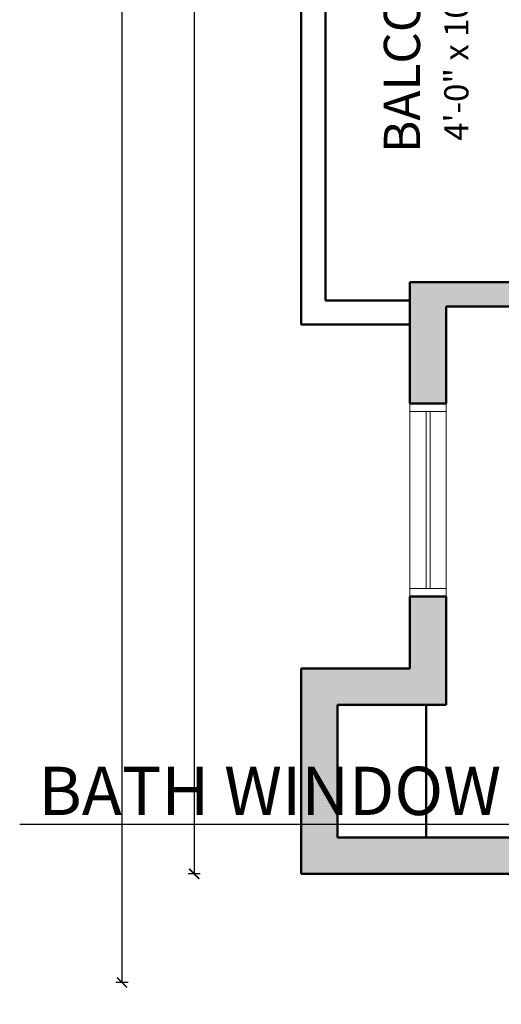
# Model space of a CAD drawing. Units: inches. Extents: x 375 to 1122, y 27 to 1069.
# Tile 2 of 155: x 375 to 494, y 155 to 400. Entities that reach past the tile are written whole.
import ezdxf

# ---------------------------------------------------------------- set-up
doc = ezdxf.new("R2010")
doc.units = ezdxf.units.IN
for name, color, linetype, lineweight in [('A-ANNO-DIMS', 2, 'Continuous', 18), ('A-AREA-IDEN', 7, 'Continuous', 18), ('A-WALL-PATT', 252, 'Continuous', 13), ('Walls', 250, 'Continuous', 50), ('Windows', 122, 'Continuous', 18)]:
    doc.layers.add(name, color=color, linetype=linetype, lineweight=lineweight)
doc.styles.get("Standard").update_dxf_attribs({"font": 'arial.ttf'})
doc.dimstyles.new('ISO-25', dxfattribs={"dimtxt": 12, "dimasz": 2.5, "dimexe": 1.5, "dimexo": 1.5, "dimtad": 1, "dimdec": 1, "dimlunit": 3, "dimtxsty": 'Standard', "dimblk": 'ARCHTICK', "dimcen": 2.5, "dimadec": 0, "dimazin": 0, "dimtfac": 1, "dimtdec": 1, "dimtmove": 0, "dimatfit": 3, "dimfxl": 1.5, "dimfxlon": 1, "dimarcsym": 0})

# ---------------------------------------------------------------- blocks, each defined once
blk = doc.blocks.new('_ArchTick')
at = {"color": 0, "linetype": 'ByBlock', "const_width": 0.15}
blk.add_lwpolyline([(-0.5, -0.5), (0.5, 0.5)], dxfattribs=at)
blk = doc.blocks.new('*D28')
at = {"layer": 'A-ANNO-DIMS', "color": 0, "lineweight": -2, "transparency": 16777216}
for p, q in [((419.42, 982.53), (416.42, 982.53)), ((417.92, 982.53), (417.92, 187.53)), ((419.42, 187.53), (416.42, 187.53))]:
    blk.add_line(p, q, dxfattribs=at)
at = {"layer": 'Defpoints', "color": 0, "transparency": 16777216}
for p in [(444.51, 982.53), (417.92, 187.53), (444.51, 187.53)]:
    blk.add_point(p, dxfattribs=at)
at = {"layer": 'A-ANNO-DIMS', "color": 0, "lineweight": -2, "transparency": 16777216, "xscale": 2.5, "yscale": 2.5, "zscale": 2.5}
for p, rotation in [((417.92, 982.53), 90), ((417.92, 187.53), 270)]:
    blk.add_blockref('_ArchTick', p, dxfattribs=dict(at, rotation=rotation))
at = {"layer": 'A-ANNO-DIMS', "color": 0, "transparency": 16777216, "insert": (411.17, 585.03), "char_height": 12, "attachment_point": 5, "rotation": 90}
blk.add_mtext('66\'-3"', dxfattribs=at)
blk = doc.blocks.new('WINDOW-48IN')
for p, q in [((2, 5), (46, 5)), ((2, 4), (46, 4))]:
    blk.add_line(p, q)
blk.add_lwpolyline([(48, 0), (0, 0), (0, 9), (48, 9)], close=True)
for points in [[(2, 0), (2, 9)], [(46, 9), (46, 0)]]:
    blk.add_lwpolyline(points)
blk = doc.blocks.new('*D49')
at = {"layer": 'A-ANNO-DIMS', "color": 0, "lineweight": -2, "transparency": 16777216}
for p, q in [((606.51, 198.25), (606.51, 201.25)), ((628.01, 198.25), (628.01, 201.25)), ((606.51, 199.75), (374.6, 199.75)), ((628.01, 199.75), (606.51, 199.75))]:
    blk.add_line(p, q, dxfattribs=at)
at = {"layer": 'Defpoints', "color": 0, "transparency": 16777216}
for p in [(606.51, 199.75), (606.51, 196.53), (628.01, 196.53)]:
    blk.add_point(p, dxfattribs=at)
at = {"layer": 'A-ANNO-DIMS', "color": 0, "lineweight": -2, "transparency": 16777216, "xscale": 2.5, "yscale": 2.5, "zscale": 2.5, "rotation": 180}
blk.add_blockref('_ArchTick', (606.51, 199.75), dxfattribs=at)
at = {"layer": 'A-ANNO-DIMS', "color": 0, "lineweight": -2, "transparency": 16777216, "xscale": 2.5, "yscale": 2.5, "zscale": 2.5}
blk.add_blockref('_ArchTick', (628.01, 199.75), dxfattribs=at)
at = {"layer": 'A-ANNO-DIMS', "color": 0, "transparency": 16777216, "insert": (489.3, 206.59), "char_height": 12, "attachment_point": 5}
blk.add_mtext('BATH WINDOW 1\'-9 1/2" TYP.', dxfattribs=at)
blk = doc.blocks.new('*D71')
at = {"layer": 'A-ANNO-DIMS', "color": 0, "lineweight": -2, "transparency": 16777216}
for p, q in [((520.11, 444.53), (520.11, 661.17)), ((518.61, 444.53), (521.61, 444.53)), ((520.11, 360.53), (520.11, 444.53)), ((518.61, 360.53), (521.61, 360.53))]:
    blk.add_line(p, q, dxfattribs=at)
at = {"layer": 'Defpoints', "color": 0, "transparency": 16777216}
for p in [(507.51, 444.53), (520.11, 444.53), (507.51, 360.53)]:
    blk.add_point(p, dxfattribs=at)
at = {"layer": 'A-ANNO-DIMS', "color": 0, "lineweight": -2, "transparency": 16777216, "xscale": 2.5, "yscale": 2.5, "zscale": 2.5}
for p, rotation in [((520.11, 444.53), 90), ((520.11, 360.53), 270)]:
    blk.add_blockref('_ArchTick', p, dxfattribs=dict(at, rotation=rotation))
at = {"layer": 'A-ANNO-DIMS', "color": 0, "transparency": 16777216, "insert": (513.27, 554.1), "char_height": 12, "attachment_point": 5, "rotation": 90}
blk.add_mtext('3-PANEL SLIDER 7\'-0" TYP.', dxfattribs=at)
blk = doc.blocks.new('*D81')
at = {"layer": 'A-ANNO-DIMS', "color": 0, "lineweight": -2, "transparency": 16777216}
for p, q in [((444.51, 117.53), (444.51, 114.53)), ((989.01, 117.53), (989.01, 114.53)), ((444.51, 116.03), (989.01, 116.03))]:
    blk.add_line(p, q, dxfattribs=at)
at = {"layer": 'Defpoints', "color": 0, "transparency": 16777216}
for p in [(444.51, 187.53), (989.01, 187.53), (989.01, 116.03)]:
    blk.add_point(p, dxfattribs=at)
at = {"layer": 'A-ANNO-DIMS', "color": 0, "lineweight": -2, "transparency": 16777216, "xscale": 2.5, "yscale": 2.5, "zscale": 2.5, "rotation": 180}
blk.add_blockref('_ArchTick', (444.51, 116.03), dxfattribs=at)
at = {"layer": 'A-ANNO-DIMS', "color": 0, "lineweight": -2, "transparency": 16777216, "xscale": 2.5, "yscale": 2.5, "zscale": 2.5}
blk.add_blockref('_ArchTick', (989.01, 116.03), dxfattribs=at)
at = {"layer": 'A-ANNO-DIMS', "color": 0, "transparency": 16777216, "insert": (716.76, 122.86), "char_height": 12, "attachment_point": 5}
blk.add_mtext('45\'-4 1/2"', dxfattribs=at)
blk = doc.blocks.new('*D82')
at = {"layer": 'A-ANNO-DIMS', "color": 0, "lineweight": -2, "transparency": 16777216}
for p, q in [((401.51, 1009.53), (398.51, 1009.53)), ((400.01, 160.53), (400.01, 1009.53)), ((401.51, 160.53), (398.51, 160.53))]:
    blk.add_line(p, q, dxfattribs=at)
at = {"layer": 'Defpoints', "color": 0, "transparency": 16777216}
for p in [(400.01, 1009.53), (630.53, 1009.53), (630.53, 160.53)]:
    blk.add_point(p, dxfattribs=at)
at = {"layer": 'A-ANNO-DIMS', "color": 0, "lineweight": -2, "transparency": 16777216, "xscale": 2.5, "yscale": 2.5, "zscale": 2.5}
for p, rotation in [((400.01, 1009.53), 90), ((400.01, 160.53), 270)]:
    blk.add_blockref('_ArchTick', p, dxfattribs=dict(at, rotation=rotation))
at = {"layer": 'A-ANNO-DIMS', "color": 0, "transparency": 16777216, "insert": (393.26, 585.03), "char_height": 12, "attachment_point": 5, "rotation": 90}
blk.add_mtext('70\'-9"', dxfattribs=at)

msp = doc.modelspace()

# ---------------------------------------------------------------- hatches: boundary and pattern name
at = {"layer": 'A-WALL-PATT'}
h = msp.add_hatch(color=256, dxfattribs=at)
h.dxf.hatch_style = 1
h.paths.add_polyline_path([(962.01, 388.53), (989.01, 388.53), (989.01, 394.53), (962.01, 394.53), (932.01, 394.53), (932.01, 397.53), (923.01, 397.53), (923.01, 394.53), (842.01, 394.53), (842.01, 334.53), (839.51, 334.53), (839.51, 328.53), (854.01, 328.53), (854.01, 334.53), (848.01, 334.53), (848.01, 388.53), (953.01, 388.53), (953.01, 356.08), (962.01, 356.08), (962.01, 358.55), (989.01, 358.55), (989.01, 364.55), (962.01, 364.55)])
h.paths.add_polyline_path([(989.01, 502.53), (932.01, 502.53), (932.01, 583.53), (932.01, 593.53), (923.01, 593.53), (923.01, 583.53), (854.01, 583.53), (854.01, 556.53), (863.01, 556.53), (863.01, 574.53), (923.01, 574.53), (923.01, 502.53), (863.01, 502.53), (863.01, 520.53), (854.01, 520.53), (854.01, 502.53), (773.01, 502.53), (773.01, 493.53), (788.01, 493.53), (788.01, 402.03), (722.01, 402.03), (722.01, 373.53), (728.01, 373.53), (728.01, 396.03), (788.01, 396.03), (788.01, 373.53), (794.01, 373.53), (794.01, 430.53), (814.01, 430.53), (814.01, 436.53), (794.01, 436.53), (794.01, 493.53), (923.01, 493.53), (923.01, 487.53), (932.01, 487.53), (932.01, 493.53), (983.01, 493.53), (983.01, 473.53), (989.01, 473.53)])
h.paths.add_polyline_path([(797.01, 325.53), (805.01, 325.53), (805.01, 328.53), (807.51, 328.53), (807.51, 334.53), (791.01, 334.53), (791.01, 226.53), (770.76, 226.53), (770.76, 217.53), (791.01, 217.53), (791.01, 187.53), (855.01, 187.53), (855.01, 196.53), (797.01, 196.53)])
h.paths.add_polyline_path([(989.01, 238.53), (962.01, 238.53), (962.01, 256.42), (953.01, 256.42), (953.01, 229.53), (980.01, 229.53), (980.01, 196.53), (915.01, 196.53), (915.01, 187.53), (989.01, 187.53)])
h.paths.add_polyline_path([(962.01, 334.53), (884.01, 334.53), (884.01, 328.53), (918.01, 328.53), (918.01, 325.53), (932.01, 325.53), (932.01, 328.53), (953.01, 328.53), (953.01, 304.42), (962.01, 304.42)])
h.paths.add_polyline_path([(606.51, 283.53), (609.51, 283.53), (609.51, 289.53), (600.51, 289.53), (600.51, 196.53), (578.51, 196.53), (578.51, 187.53), (606.51, 187.53), (606.51, 196.53)])
h.paths.add_polyline_path([(666.51, 292.53), (660.51, 292.53), (660.51, 289.53), (633.51, 289.53), (633.51, 283.53), (660.51, 283.53), (660.51, 196.53), (628.01, 196.53), (628.01, 187.53), (630.53, 187.53), (630.53, 160.53), (636.53, 160.53), (636.53, 187.53), (660.51, 187.53), (660.51, 160.53), (666.51, 160.53), (666.51, 217.53), (686.76, 217.53), (686.76, 226.53), (666.51, 226.53)])
h.paths.add_polyline_path([(480.51, 256.42), (471.51, 256.42), (471.51, 238.53), (444.51, 238.53), (444.51, 187.53), (518.51, 187.53), (518.51, 196.53), (453.51, 196.53), (453.51, 229.53), (480.51, 229.53)])
h.paths.add_polyline_path([(480.51, 328.53), (652.51, 328.53), (652.51, 325.53), (660.51, 325.53), (660.51, 322.53), (666.51, 322.53), (666.51, 334.53), (507.51, 334.53), (507.51, 360.53), (498.51, 360.53), (498.51, 334.53), (471.51, 334.53), (471.51, 304.42), (480.51, 304.42)])
h.paths.add_polyline_path([(507.51, 484.53), (498.51, 484.53), (498.51, 444.53), (507.51, 444.53), (507.51, 454.53), (621.51, 454.53), (621.51, 460.53), (507.51, 460.53)])
h.paths.add_polyline_path([(672.51, 604.53), (683.26, 604.53), (683.26, 613.53), (669.51, 613.53), (669.51, 649.53), (663.51, 649.53), (663.51, 589.53), (507.51, 589.53), (507.51, 613.53), (498.51, 613.53), (498.51, 556.53), (507.51, 556.53), (507.51, 580.53), (663.51, 580.53), (663.51, 520.53), (669.51, 520.53), (669.51, 556.53), (683.26, 556.53), (683.26, 565.53), (672.51, 565.53)])
h.paths.add_polyline_path([(731.01, 667.53), (734.01, 667.53), (734.01, 676.53), (728.01, 676.53), (728.01, 715.53), (657.51, 715.53), (657.51, 709.53), (663.51, 709.53), (663.51, 673.53), (669.51, 673.53), (669.51, 709.53), (722.01, 709.53), (722.01, 613.53), (704.76, 613.53), (704.76, 604.53), (722.01, 604.53), (722.01, 565.53), (704.76, 565.53), (704.76, 556.53), (722.01, 556.53), (722.01, 502.53), (722.01, 460.53), (669.51, 460.53), (669.51, 496.53), (663.51, 496.53), (663.51, 460.53), (657.51, 460.53), (657.51, 454.53), (728.01, 454.53), (728.01, 493.53), (734.01, 493.53), (734.01, 502.53), (731.01, 502.53)])
h.paths.add_polyline_path([(986.01, 718.53), (959.01, 718.53), (959.01, 727.53), (950.01, 727.53), (950.01, 709.53), (977.01, 709.53), (977.01, 676.53), (794.01, 676.53), (794.01, 805.53), (802.01, 805.53), (802.01, 808.53), (804.51, 808.53), (804.51, 814.53), (788.01, 814.53), (788.01, 774.03), (728.01, 774.03), (728.01, 796.53), (722.01, 796.53), (722.01, 768.03), (788.01, 768.03), (788.01, 676.53), (773.01, 676.53), (773.01, 667.53), (923.01, 667.53), (923.01, 657.53), (932.01, 657.53), (932.01, 667.53), (986.01, 667.53)])
h.paths.add_polyline_path([(621.51, 715.53), (507.51, 715.53), (507.51, 733.53), (498.51, 733.53), (498.51, 715.53), (498.51, 685.53), (507.51, 685.53), (507.51, 709.53), (621.51, 709.53)])
h.paths.add_polyline_path([(666.51, 847.03), (660.51, 847.03), (660.51, 844.53), (652.51, 844.53), (652.51, 841.53), (480.51, 841.53), (480.51, 859.53), (471.51, 859.53), (471.51, 835.53), (498.51, 835.53), (498.51, 817.53), (507.51, 817.53), (507.51, 835.53), (666.51, 835.53)])
h.paths.add_polyline_path([(480.51, 940.53), (453.51, 940.53), (453.51, 973.53), (518.51, 973.53), (518.51, 982.53), (444.51, 982.53), (444.51, 931.53), (471.51, 931.53), (471.51, 907.53), (480.51, 907.53)])
h.paths.add_polyline_path([(606.51, 982.53), (578.51, 982.53), (578.51, 973.53), (600.51, 973.53), (600.51, 880.53), (609.51, 880.53), (609.51, 886.53), (606.51, 886.53)])
h.paths.add_polyline_path([(666.51, 943.53), (686.76, 943.53), (686.76, 952.53), (666.51, 952.53), (666.51, 1009.53), (660.51, 1009.53), (660.51, 982.53), (636.53, 982.53), (636.53, 1009.53), (630.53, 1009.53), (630.53, 982.53), (628.01, 982.53), (628.01, 973.53), (660.51, 973.53), (660.51, 886.53), (633.51, 886.53), (633.51, 880.53), (660.51, 880.53), (660.51, 877.03), (666.51, 877.03)])
h.paths.add_polyline_path([(986.01, 874.53), (932.01, 874.53), (932.01, 877.53), (923.01, 877.53), (923.01, 874.53), (788.01, 874.53), (788.01, 868.53), (788.01, 844.53), (794.01, 844.53), (794.01, 868.53), (839.01, 868.53), (839.01, 814.53), (836.51, 814.53), (836.51, 808.53), (851.01, 808.53), (851.01, 814.53), (845.01, 814.53), (845.01, 868.53), (986.01, 868.53)])
h.paths.add_polyline_path([(959.01, 838.55), (986.01, 838.55), (986.01, 844.55), (959.01, 844.55), (959.01, 847.03), (950.01, 847.03), (950.01, 814.53), (881.01, 814.53), (881.01, 808.53), (918.01, 808.53), (918.01, 805.53), (932.01, 805.53), (932.01, 808.53), (950.01, 808.53), (950.01, 793.53), (959.01, 793.53)])
h.paths.add_polyline_path([(986.01, 982.53), (899.01, 982.53), (899.01, 973.53), (923.01, 973.53), (923.01, 967.53), (932.01, 967.53), (932.01, 973.53), (980.01, 973.53), (980.01, 953.53), (986.01, 953.53)])
h.paths.add_polyline_path([(851.01, 982.53), (788.01, 982.53), (788.01, 952.53), (770.76, 952.53), (770.76, 943.53), (788.01, 943.53), (788.01, 910.53), (814.01, 910.53), (814.01, 916.53), (794.01, 916.53), (794.01, 973.53), (851.01, 973.53)])

# ---------------------------------------------------------------- linework, layer by layer
at = {"layer": 'Walls'}
for p, q in [((444.51, 324.03), (444.51, 465.03)), ((450.51, 330.03), (450.51, 459.03)), ((471.51, 334.53), (498.51, 334.53)), ((471.51, 304.42), (471.51, 334.53)), ((450.51, 330.03), (471.51, 330.03)), ((480.51, 328.53), (652.51, 328.53)), ((480.51, 304.42), (480.51, 328.53)), ((444.51, 324.03), (471.51, 324.03)), ((480.51, 304.42), (471.51, 304.42)), ((471.51, 238.53), (471.51, 256.42)), ((480.51, 256.42), (471.51, 256.42)), ((480.51, 229.53), (480.51, 256.42)), ((444.51, 187.53), (444.51, 238.53)), ((444.51, 238.53), (471.51, 238.53)), ((453.51, 229.53), (480.51, 229.53)), ((453.51, 196.53), (453.51, 229.53)), ((475.51, 196.53), (475.51, 229.53)), ((518.51, 196.53), (453.51, 196.53)), ((444.51, 187.53), (518.51, 187.53))]:
    msp.add_line(p, q, dxfattribs=at)

# ---------------------------------------------------------------- block references
at = {"layer": 'Windows', "rotation": 270}
msp.add_blockref('WINDOW-48IN', (471.51, 304.42), dxfattribs=at)

# ---------------------------------------------------------------- texts
at = {"layer": 'A-AREA-IDEN', "insert": (465.03, 360.85), "char_height": 12, "attachment_point": 1, "rotation": 90}
msp.add_mtext_dynamic_manual_height_columns('\\pxqc;{\\fArial|b1|i0|c0|p34;\\H0.75x;BALCONY\\H1.33333x;\\P\\fArial|b0|i0|c0|p34;\\H0.5x;4\'-0" x 10\'-9"}', width=66.1169, gutter_width=12.5, heights=[0], dxfattribs=at)

# ---------------------------------------------------------------- dimensions: what is measured, and where the dimension line sits
at = {"layer": 'A-ANNO-DIMS'}
for base, p1, p2, override, picture, middle in [((400.01, 1009.53), (630.53, 160.53), (630.53, 1009.53), {"dimdec": 1, "dimlfac": 1, "dimrnd": 0, "dimzin": 1, "dimdsep": 46, "dimlunit": 4, "dimfrac": 2}, '*D82', (393.26, 585.03)), ((417.92, 187.53), (444.51, 982.53), (444.51, 187.53), {"dimclrd": 0, "dimclre": 0, "dimclrt": 0}, '*D28', (411.17, 585.03))]:
    dim = msp.add_linear_dim(base=base, p1=p1, p2=p2, angle=90, dimstyle='ISO-25', override=override, dxfattribs=at)
    dim.commit()
    dim.dimension.update_dxf_attribs({"geometry": picture, "text_midpoint": middle})
for base, p1, p2, angle, text, picture, middle in [((520.11, 444.53), (507.51, 360.53), (507.51, 444.53), 90, '3-PANEL SLIDER <> TYP.', '*D71', (513.27, 554.1)), ((606.51, 199.75), (628.01, 196.53), (606.51, 196.53), 180, 'BATH WINDOW <> TYP.', '*D49', (489.3, 206.59))]:
    dim = msp.add_linear_dim(base=base, p1=p1, p2=p2, angle=angle, text=text, dimstyle='ISO-25', override={"dimdec": 1, "dimlfac": 1, "dimrnd": 0, "dimzin": 1, "dimdsep": 46, "dimlunit": 4, "dimfrac": 2}, dxfattribs=at)
    dim.commit()
    dim.dimension.update_dxf_attribs({"geometry": picture, "text_midpoint": middle})
dim = msp.add_linear_dim(base=(989.01, 116.03), p1=(444.51, 187.53), p2=(989.01, 187.53), dimstyle='ISO-25', override={"dimdec": 1, "dimlfac": 1, "dimrnd": 0, "dimzin": 1, "dimdsep": 46, "dimlunit": 4, "dimfrac": 2}, dxfattribs=at)
dim.commit()
dim.dimension.update_dxf_attribs({"geometry": '*D81', "text_midpoint": (716.76, 122.86)})

doc.saveas('drawing.dxf')
